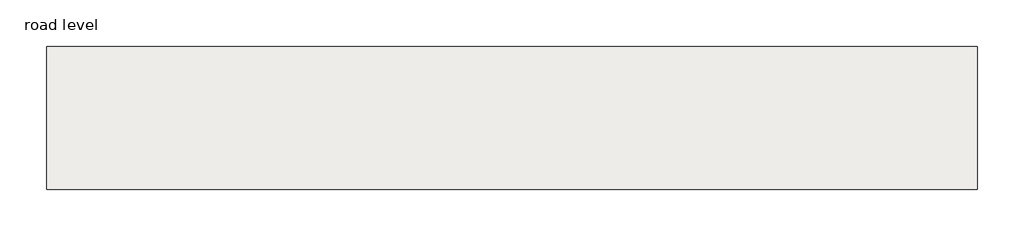
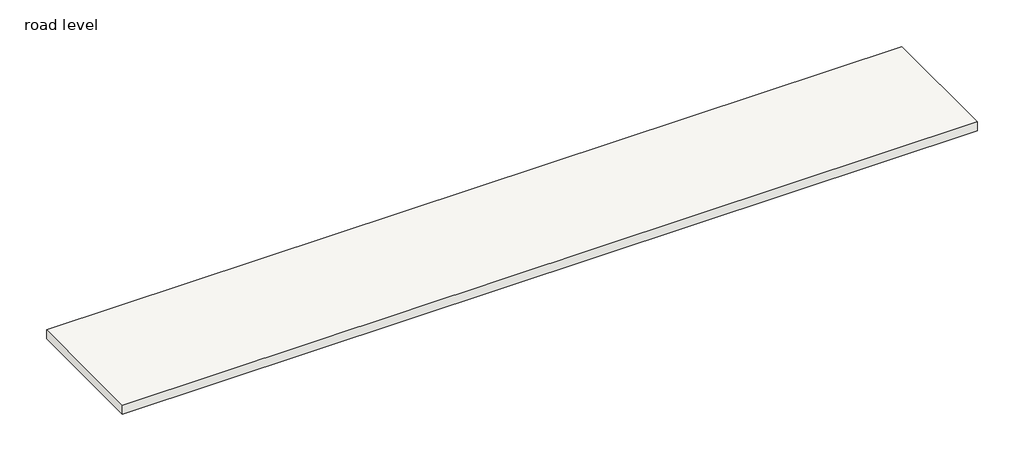
# One storey: 1 slab.
"""IFC4 building model written with IfcOpenShell, lengths in millimetres."""

from ifc_helpers import new_model, si_unit, frame, origin, place, context, project, spatial, polyline, outline, extrude, element, save

model = new_model("IFC4")

# Units and contexts
model_context = context("Model", 3, world=origin())
ifc_project = project(units=[si_unit("LENGTHUNIT", "METRE", prefix="MILLI")], contexts=[model_context])

# Site, building, storey
site = spatial("IfcSite", under=ifc_project)
building = spatial("IfcBuilding", under=site)
storey = spatial("IfcBuildingStorey", under=building, Name="road level", Elevation=0.0)

# Slab
placement = place(None, origin())
element("IfcSlab", 1, ObjectType="Generic - 12\"", at=placement, inside=storey, context=model_context, shape_type="SweptSolid", body=[
    extrude(outline(polyline([(-16496.9544965, -12287.0518998), (-16496.9544965, -8070.6518998), (10935.0455035, -8070.6518998), (10935.0455035, -12287.0518998), (-16496.9544965, -12287.0518998)])), frame((0.0, 0.0, -304.8), z_axis=(0.0, 0.0, 1.0), x_axis=(1.0, 0.0, 0.0)), (0.0, 0.0, 1.0), 304.8),
])

save(model, "model.ifc")

# Revit data of these elements
# Type "Generic - 12\""
#   Assembly Code = "B1010"
#   Function = 0
#   Layers, outside or top first: 1' - 0" "black metal" (function 1)
# Element 1 (IfcSlab, "Generic - 12\"")
#   built-in parameter 1001955 = -1.5708 (stored number, unit not read)
#   Height Offset From Level = 0' - 0"
#   Phase Created = New Construction
#   Materials on its faces: "black metal"
# Materials
#   "black metal": class "Generic", colour RGB 120 120 120, transparency 0, Cost = 0
